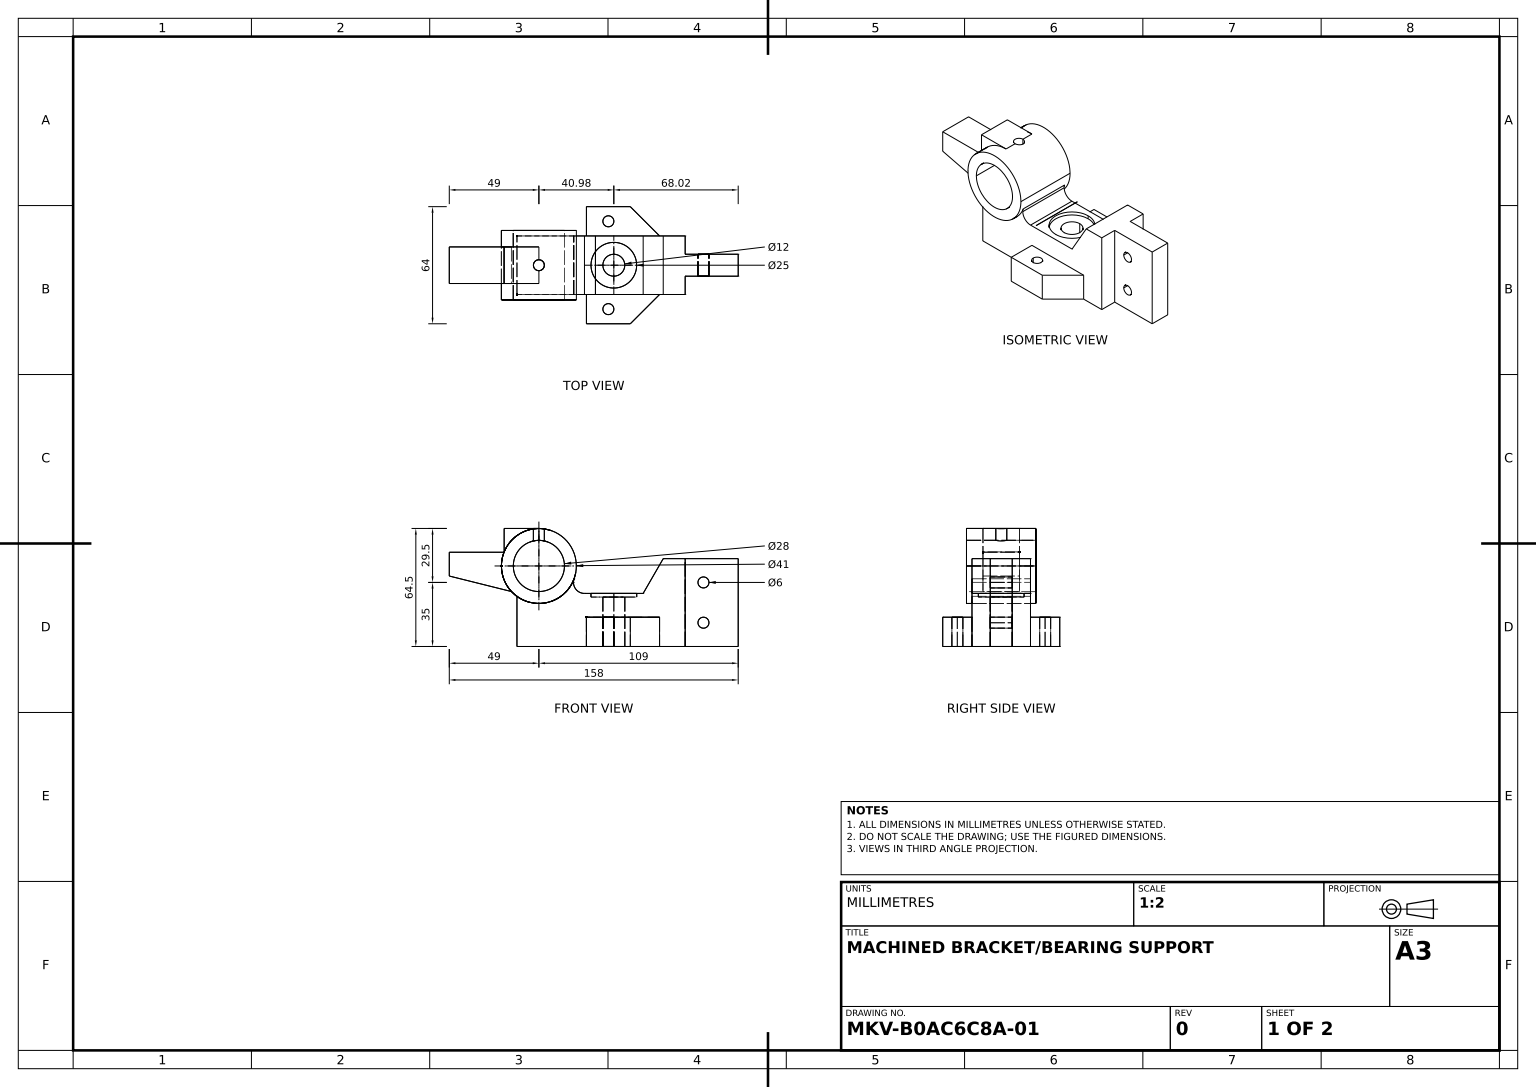
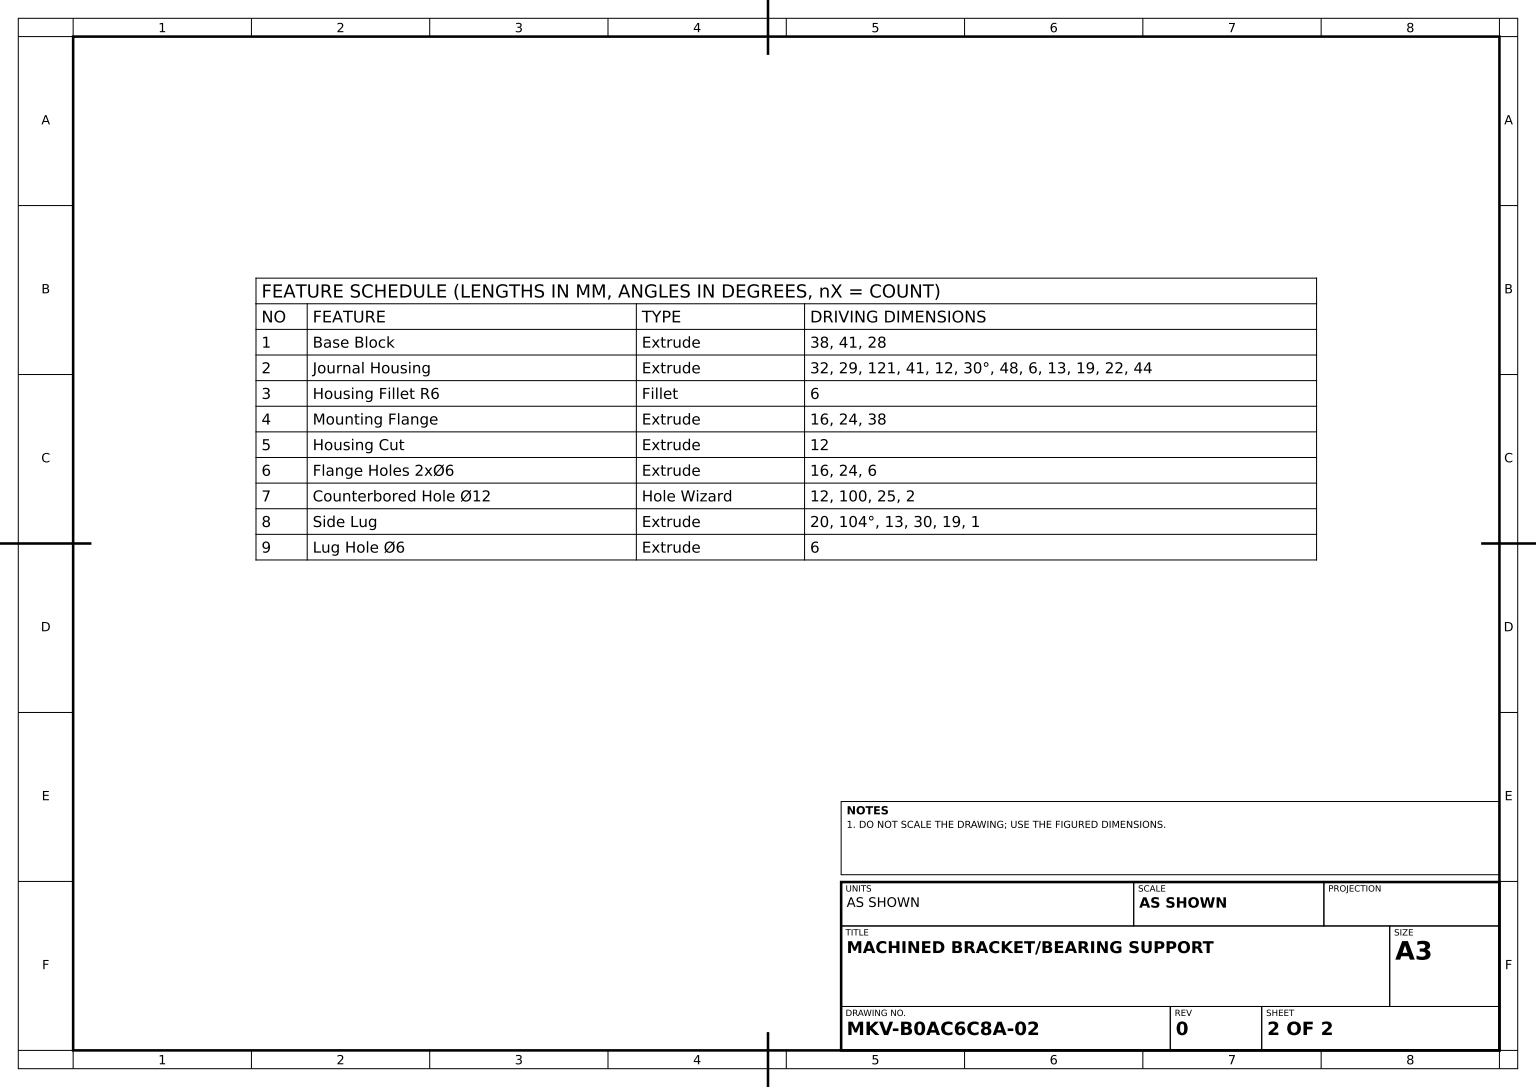
from build123d import *

# Parameters (mm, degrees)
BASE_BLOCK_SKETCH_R              = 20.5
BASE_BLOCK_SKETCH_R_2            = 14
BASE_BLOCK_DEPTH                 = 19
JOURNAL_HOUSING_PROFILE_SKETCH_R = 3
JOURNAL_HOUSING_DEPTH            = 16
HOUSING_FILLET_R6_R              = 6
MOUNTING_FLANGE_DEPTH            = 16
HOUSING_CUT_SKETCH_W             = 29
HOUSING_CUT_SKETCH_H             = 10
HOUSING_CUT_DEPTH                = 124.324774478
FLANGE_HOLES_SKETCH_R            = 3
FLANGE_HOLES_2X_6_DEPTH          = 16
COUNTERBORED_HOLE_12_D           = 12
COUNTERBORED_HOLE_12_DEPTH       = 99.788526395
COUNTERBORED_HOLE_12_CBORE_D     = 25
COUNTERBORED_HOLE_12_CBORE_DEPTH = 2
SIDE_LUG_DEPTH                   = 10
LUG_HOLE_6_REACH                 = 132.634
LUG_HOLE_6_END_RADIUS            = 14
LUG_HOLE_SKETCH_R                = 3


with BuildPart() as part:
    # Base Block Sketch → Base Block (new, symmetric)
    with BuildSketch(Plane.XY):
        Circle(BASE_BLOCK_SKETCH_R)
        Circle(BASE_BLOCK_SKETCH_R_2, mode=Mode.SUBTRACT)
    extrude(amount=BASE_BLOCK_DEPTH, both=True)

    # Journal Housing Profile Sketch → Journal Housing (add, symmetric)
    with BuildSketch(Plane.XY):
        Polygon((-12, -44), (-12, -15), (57.030344885, -15), (68, 4), (109, 4), (109, -44), align=None)
        with Locations((90, -31)):
            Circle(JOURNAL_HOUSING_PROFILE_SKETCH_R, mode=Mode.SUBTRACT)
        with Locations((90, -9)):
            Circle(JOURNAL_HOUSING_PROFILE_SKETCH_R, mode=Mode.SUBTRACT)
    extrude(amount=JOURNAL_HOUSING_DEPTH, both=True)

    # Housing Fillet R6
    housing_fillet_r6_edges = [part.edges().sort_by_distance(p)[0] for p in [
        (13.973188612, -15, 0),
    ]]
    fillet(housing_fillet_r6_edges, radius=HOUSING_FILLET_R6_R)

    # Mounting Flange Sketch → Mounting Flange (add)
    with BuildSketch(Plane.XZ.offset(44)):
        Polygon((26, 16), (26, 32), (50, 32), (66, 16), align=None)
        Polygon((50, -32), (66, -16), (26, -16), (26, -32), align=None)
    extrude(amount=-MOUNTING_FLANGE_DEPTH)

    # Housing Cut Sketch → Housing Cut (cut, through all)
    with BuildSketch(Plane(origin=(0, 4, 0), x_dir=(1, 0, 0), z_dir=(0, 1, 0))):
        with Locations((94.5, -11)):
            Rectangle(HOUSING_CUT_SKETCH_W, HOUSING_CUT_SKETCH_H)
        with Locations((94.5, 11)):
            Rectangle(HOUSING_CUT_SKETCH_W, HOUSING_CUT_SKETCH_H)
    extrude(amount=-HOUSING_CUT_DEPTH, mode=Mode.SUBTRACT)

    # Flange Holes Sketch → Flange Holes 2xØ6 (cut)
    with BuildSketch(Plane(origin=(0, -28, 0), x_dir=(1, 0, 0), z_dir=(0, 1, 0))):
        with Locations(Location((38, -24, 0), (0, 0, 180))):
            Circle(FLANGE_HOLES_SKETCH_R)
        with Locations((38, 24)):
            Circle(FLANGE_HOLES_SKETCH_R)
    extrude(amount=-FLANGE_HOLES_2X_6_DEPTH, mode=Mode.SUBTRACT)

    # Counterbored Hole Ø12
    with Locations(Plane(origin=(40.977616023, -15, 0), x_dir=(0, 0, 1), z_dir=(0, 1, 0))):
        with Locations((0, 0)):
            CounterBoreHole(COUNTERBORED_HOLE_12_D / 2, COUNTERBORED_HOLE_12_CBORE_D / 2, COUNTERBORED_HOLE_12_CBORE_DEPTH, depth=COUNTERBORED_HOLE_12_DEPTH)

    # Side Lug Sketch → Side Lug (add, symmetric)
    with BuildSketch(Plane.XY):
        with BuildLine():
            Line((0, 20.5), (-19, 20.5))
            Line((-19, 20.5), (-19, 7.5))
            Line((-19, 7.5), (-49, 7.5))
            Line((-49, 7.5), (-49, -5.5))
            Line((-49, -5.5), (-13.090107344, -14.453341818))
            ThreePointArc((-13.090107344, -14.453341818), (-18.194644342, 7.014621677), (0, 19.5))
            Line((0, 19.5), (0, 20.5))
        make_face()
    extrude(amount=SIDE_LUG_DEPTH, both=True)

    # Lug Hole Ø6: up to this cylinder (the profile starts outside it)
    lug_hole_6_end = Plane(origin=(0, 0, 0), z_dir=(0, 0, -1)) * Cylinder(LUG_HOLE_6_END_RADIUS, 294.268, mode=Mode.PRIVATE)
    # Lug Hole Sketch → Lug Hole Ø6 (cut, up to the surface)
    with BuildSketch(Plane(origin=(0, 20.5, 0), x_dir=(1, 0, 0), z_dir=(0, 1, 0)), mode=Mode.PRIVATE) as lug_hole_6_sk1:
        with Locations(Location((0, 0, 0), (0, 0, 270))):
            Circle(LUG_HOLE_SKETCH_R)
    lug_hole_6_tool1 = extrude(lug_hole_6_sk1.sketch, amount=-LUG_HOLE_6_REACH, mode=Mode.PRIVATE) - lug_hole_6_end
    add(lug_hole_6_tool1.solids().sort_by_distance((0, 20.5, 0))[0], mode=Mode.SUBTRACT)


solid = part.part
